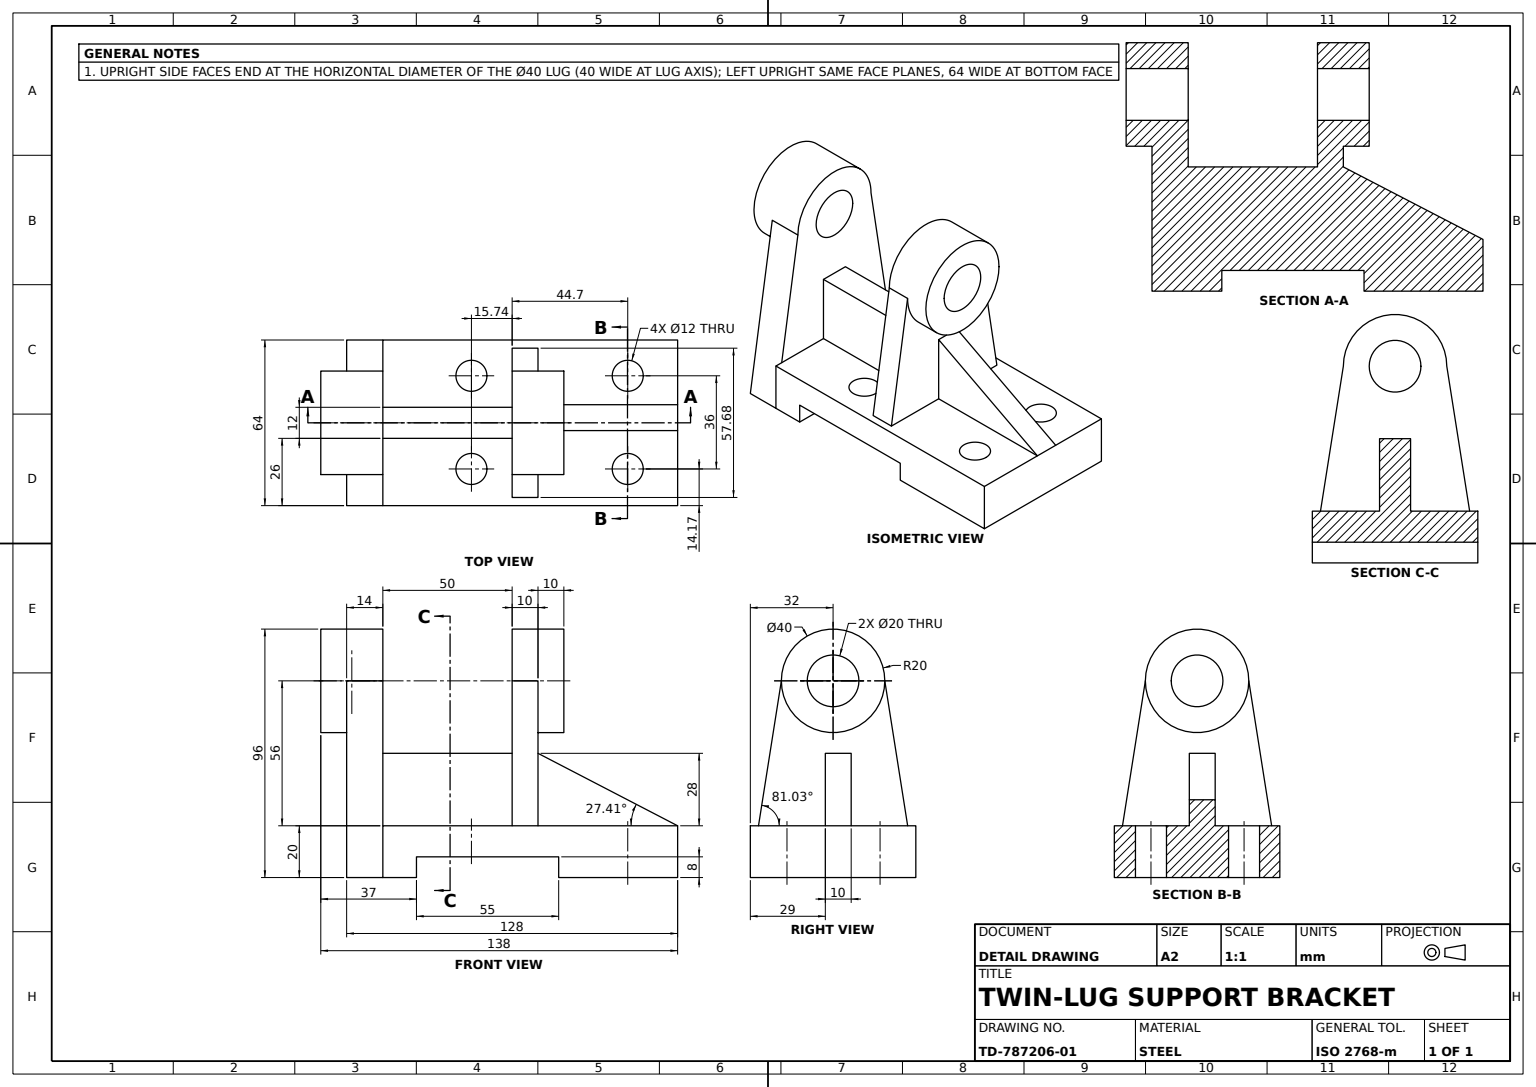
SolidWorks part; units mm, degrees
material "Plain Carbon Steel"
ref_plane "Front Plane" through (0, 0, 0) normal (0, 0, 1) x (1, 0, 0)
ref_plane "Top Plane" through (0, 0, 0) normal (0, 1, 0) x (1, 0, 0)
ref_plane "Right Plane" through (0, 0, 0) normal (1, 0, 0) x (0, 0, -1)
sketch "Base Profile Sketch" plane through (0, 0, 0) normal (0, 0, 1) x (1, 0, 0)
  line L1 (-64, 10) -> (64, 10)
  line L2 (-64, 10) -> (-64, -10)
  line L3 (-64, -10) -> (64, -10)
  line L4 (64, 10) -> (64, -10)
  line L5 (-64, 10) -> (64, -10) construction
  line L6 (-64, -10) -> (64, 10) construction
  point P0 (0, 0)
  dimension "D1" = 20
  dimension "D2" = 128
extrude "Base Plate" add sketch "Base Profile Sketch" along normal blind 64
sketch "Underside Relief Sketch" plane through (0, 0, 0) normal (0, 0, 1) x (1, 0, 0)
  line L1 (-64, -10) -> (64, -10) construction
  line L2 (-37, -10) -> (-37, -2)
  line L3 (-37, -2) -> (18, -2)
  line L4 (18, -2) -> (18, -10)
  line L5 (18, -10) -> (-37, -10)
  dimension "D1" = 55
  dimension "D2" = 8
  dimension "D3" = 37
extrude "Underside Relief Cut" cut sketch "Underside Relief Sketch" against normal blind 64 and the other way through all
sketch "First Upright Sketch" plane through (0, 10, 0) normal (0, 1, 0) x (1, 0, 0)
  line L0 (64, -64) -> (-64, -64) construction
  line L1 (-64, 0) -> (-50, 0)
  line L2 (-64, 0) -> (-64, -64)
  line L3 (-64, -64) -> (-50, -64)
  line L4 (-50, 0) -> (-50, -64)
  line L5 (-64, -64) -> (-64, 0) construction
  dimension "D1" = 14
extrude "First Upright" add sketch "First Upright Sketch" along normal blind 56
sketch "First Trunnion Boss Sketch" plane through (-64, 0, 0) normal (-1, 0, 0) x (0, 0, 1)
  line L0 (0, 66) -> (64, 66) construction
  circle A0 centre (32, 66) radius 20
  circle A1 centre (32, 66) radius 10
  dimension "D1" = 20
  dimension "D2" = 40
extrude "First Trunnion Boss" add sketch "First Trunnion Boss Sketch" against normal blind 14 and the other way blind 10
sketch "First Trunnion Bore Sketch" plane through (-64, 0, 0) normal (-1, 0, 0) x (0, 0, 1)
  line L1 (42, 66) -> (22, 66)
  line L2 (42, 66) -> (22, 66)
  arc A1 (22, 66) -> (42, 66) centre (32, 66) ccw
  arc A2 (22, 66) -> (42, 66) centre (32, 66) ccw
  dimension "D1" = 0
extrude "First Trunnion Bore" cut sketch "First Trunnion Bore Sketch" against normal blind 14
sketch "First Upright Taper Sketch" plane through (-64, 0, 0) normal (-1, 0, 0) x (0, 0, 1)
  line L0 (12, 66) -> (0, -10)
  line L1 (0, -10) -> (64, -10)
  line L2 (64, -10) -> (52, 66)
  line L3 (52, 66) -> (64, 66)
  line L4 (64, 66) -> (64, -10)
  line L5 (12, 66) -> (0, 66)
  line L6 (0, 66) -> (0, -10)
  circle A0 centre (32, 66) radius 20 construction
  line M2 (12, 66) -> (0, 66)
  line M3 (0, 66) -> (0, -10)
  line M5 (64, -10) -> (64, 66)
  line M6 (64, 66) -> (52, 66)
extrude "First Upright Taper Cut" cut sketch "First Upright Taper Sketch" against normal blind 14 contours L0 M2 M3 | L2 M5 M6
sketch "Center Block Sketch" plane through (0, 10, 0) normal (0, 1, 0) x (1, 0, 0)
  line L0 (-50, -32) -> (0, -32) construction
  line L1 (-50, -60.8421) -> (-50, -3.1579) construction
  line L2 (-50, -32) -> (-50, -26)
  line L3 (-50, -52) -> (-50, -12) construction
  line L4 (-50, -26) -> (0, -26)
  line L5 (0, -26) -> (0, -38)
  line L6 (0, -38) -> (-50, -38)
  line L7 (-50, -38) -> (-50, -32)
  line L9 (64, -64) -> (-50, -64) construction
  dimension "D1" = 26
extrude "Center Block" add sketch "Center Block Sketch" along normal blind 28
sketch "Second Trunnion Boss Sketch" plane through (0, 0, 0) normal (1, 0, 0) x (0, 0, -1)
  circle A0 centre (-32, 66) radius 10
  circle A1 centre (-32, 66) radius 20
  dimension "D1" = 20
  dimension "D2" = 40
extrude "Second Trunnion Boss" add sketch "Second Trunnion Boss Sketch" along normal blind 20 separate body
sketch "Second Upright Sketch" plane through (0, 0, 0) normal (1, 0, 0) x (0, 0, -1)
  line L0 (-52, 66) -> (-60.8421, 10)
  line L1 (-60.8421, 10) -> (-3.1579, 10)
  line L2 (-3.1579, 10) -> (-12, 66)
  line L3 (-12, 66) -> (-3.1579, 10) construction
  line L4 (-52, 66) -> (-12, 66)
  circle A0 centre (-32, 66) radius 20 construction
extrude "Second Upright" add sketch "Second Upright Sketch" along normal blind 10
sketch "Second Trunnion Bore Sketch" plane through (0, 0, 0) normal (1, 0, 0) x (0, 0, -1)
  line L1 (-22, 66) -> (-42, 66)
  line L2 (-22, 66) -> (-42, 66)
  arc A1 (-42, 66) -> (-22, 66) centre (-32, 66) ccw
  arc A2 (-42, 66) -> (-22, 66) centre (-32, 66) ccw
  dimension "D1" = 0
extrude "Second Trunnion Bore" cut sketch "Second Trunnion Bore Sketch" along normal blind 10
ref_plane "Rib Plane" through (0, 0, 30) normal (0, 0, 1) x (1, 0, 0)
sketch "Gusset Rib Sketch" plane through (0, 0, 30) normal (0, 0, 1) x (1, 0, 0)
  line L0 (10, 38) -> (64, 10)
  line L1 (10, 66) -> (10, 10) construction
rib "Gusset Rib" sketch "Gusset Rib Sketch" sketch "Gusset Rib Sketch" thickness 10 extrusion direction parallel to sketch draft on no parameters "D1"=10
sketch "Base Mounting Holes Sketch" plane through (0, 10, 0) normal (0, 1, 0) x (1, 0, 0)
  line L0 (0, -26) -> (0, -3.1579) construction
  line L1 (10, -3.1579) -> (0, -3.1579) construction
  circle A0 centre (-15.7438, -13.8283) radius 6
  circle A1 centre (-15.7438, -49.8283) radius 6
  circle A2 centre (44.7041, -13.8283) radius 6
  circle A3 centre (44.7041, -49.8283) radius 6
  dimension "D1" = 12
  dimension "D2" = 44.7041
  dimension "D3" = 15.7438
  dimension "D4" = 10.6704
  dimension "D5" = 46.6704
extrude "Base Mounting Holes" cut sketch "Base Mounting Holes Sketch" against normal through all
